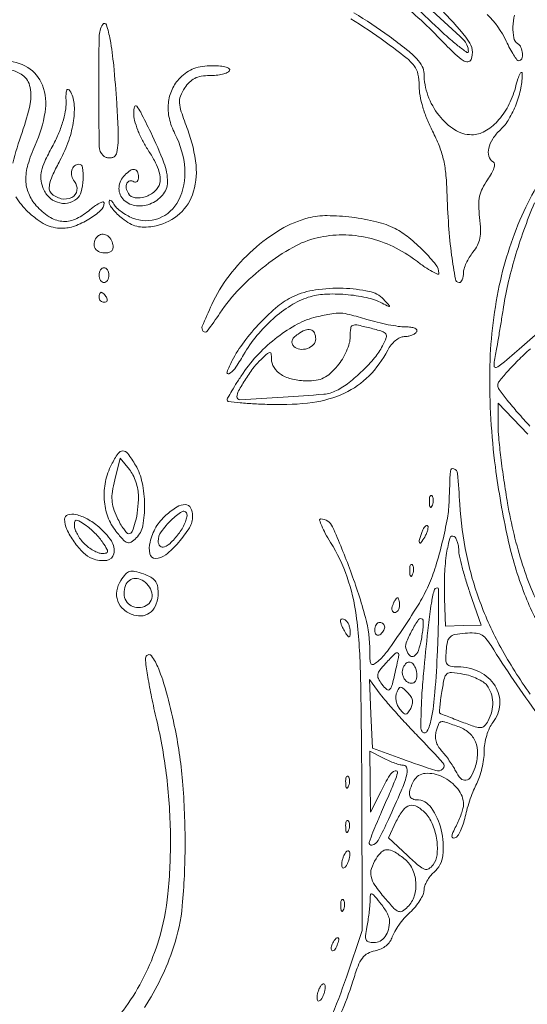
# Model space of a CAD drawing. Units: inches. Extents: x 2656 to 9931, y 1941 to 3068.
# Tile 38 of 46: x 2847 to 2854, y 2967 to 2981. Entities that reach past the tile are written whole.
import ezdxf

# ---------------------------------------------------------------- set-up
doc = ezdxf.new("R2010")
doc.units = ezdxf.units.IN
doc.layers.add('A-ANNO-DIMS', color=2, linetype='Continuous', lineweight=18)
doc.layers.add('A-ELEV-ORN', color=8, linetype='Continuous', lineweight=13)
doc.styles.get("Standard").update_dxf_attribs({"font": 'arial.ttf'})
doc.dimstyles.new('ISO-25', dxfattribs={"dimtxt": 6, "dimasz": 2.5, "dimexe": 1.25, "dimexo": 0.625, "dimtad": 1, "dimdec": 0, "dimlunit": 3, "dimtxsty": 'Standard', "dimcen": 2.5, "dimadec": 0, "dimazin": 0, "dimtfac": 1, "dimtdec": 0, "dimtmove": 0, "dimatfit": 3, "dimfxl": 1, "dimarcsym": 0})

# ---------------------------------------------------------------- blocks, each defined once
blk = doc.blocks.new('*D152')
at = {"layer": 'A-ANNO-DIMS', "color": 0, "lineweight": -2, "transparency": 16777216}
for p, q in [((2847.28, 2990.828), (2707.323, 2990.828)), ((2708.573, 2988.328), (2708.573, 2952.971)), ((2847.248, 2950.471), (2707.323, 2950.471))]:
    blk.add_line(p, q, dxfattribs=at)
at = {"layer": 'A-ANNO-DIMS', "color": 0, "transparency": 16777216}
for points in [[(2708.156, 2988.328), (2708.989, 2988.328), (2708.573, 2990.828)], [(2708.156, 2952.971), (2708.989, 2952.971), (2708.573, 2950.471)]]:
    blk.add_solid(points, dxfattribs=at)
at = {"layer": 'Defpoints', "color": 0, "transparency": 16777216}
for p in [(2847.905, 2990.828), (2708.573, 2950.471), (2847.873, 2950.471)]:
    blk.add_point(p, dxfattribs=at)
at = {"layer": 'A-ANNO-DIMS', "color": 0, "transparency": 16777216, "insert": (2704.843, 2970.649), "char_height": 6, "attachment_point": 5, "rotation": 90}
blk.add_mtext('3\'-4 1/2"', dxfattribs=at)
blk = doc.blocks.new('*D153')
at = {"layer": 'A-ANNO-DIMS', "color": 0, "lineweight": -2, "transparency": 16777216}
for p, q in [((2826.64, 2993.722), (2826.64, 2703.709)), ((2829.546, 2956.424), (2829.546, 2703.709)), ((2824.14, 2704.959), (2821.64, 2704.959)), ((2826.64, 2704.959), (2829.546, 2704.959)), ((2832.046, 2704.959), (2851.745, 2704.959))]:
    blk.add_line(p, q, dxfattribs=at)
at = {"layer": 'A-ANNO-DIMS', "color": 0, "transparency": 16777216}
for points in [[(2824.14, 2705.376), (2824.14, 2704.543), (2826.64, 2704.959)], [(2832.046, 2705.376), (2832.046, 2704.543), (2829.546, 2704.959)]]:
    blk.add_solid(points, dxfattribs=at)
at = {"layer": 'Defpoints', "color": 0, "transparency": 16777216}
for p in [(2826.64, 2994.347), (2829.546, 2957.049), (2829.546, 2704.959)]:
    blk.add_point(p, dxfattribs=at)
at = {"layer": 'A-ANNO-DIMS', "color": 0, "transparency": 16777216, "insert": (2843.145, 2708.65), "char_height": 6, "attachment_point": 5}
blk.add_mtext('0\'-3"', dxfattribs=at)
blk = doc.blocks.new('*D154')
at = {"layer": 'A-ANNO-DIMS', "color": 0, "lineweight": -2, "transparency": 16777216}
for p, q in [((2708.573, 2996.847), (2708.573, 2999.347)), ((2826.015, 2994.347), (2707.323, 2994.347)), ((2708.573, 2994.347), (2708.573, 2990.828)), ((2847.28, 2990.828), (2707.323, 2990.828)), ((2708.573, 2988.328), (2708.573, 2954.647))]:
    blk.add_line(p, q, dxfattribs=at)
at = {"layer": 'A-ANNO-DIMS', "color": 0, "transparency": 16777216}
for points in [[(2708.156, 2996.847), (2708.989, 2996.847), (2708.573, 2994.347)], [(2708.156, 2988.328), (2708.989, 2988.328), (2708.573, 2990.828)]]:
    blk.add_solid(points, dxfattribs=at)
at = {"layer": 'Defpoints', "color": 0, "transparency": 16777216}
for p in [(2826.64, 2994.347), (2708.573, 2990.828), (2847.905, 2990.828)]:
    blk.add_point(p, dxfattribs=at)
at = {"layer": 'A-ANNO-DIMS', "color": 0, "transparency": 16777216, "insert": (2704.843, 2970.237), "char_height": 6, "attachment_point": 5, "rotation": 90}
blk.add_mtext('0\'-3 1/2"', dxfattribs=at)

msp = doc.modelspace()

# ---------------------------------------------------------------- linework, layer by layer
at = {"layer": 'A-ELEV-ORN'}
for points in [[(2851.141, 2982.631, 0.234084), (2851.162, 2982.589, 0.005273), (2851.348, 2982.45, 0.010754), (2851.575, 2982.292, 0.006932), (2851.845, 2982.118, -0.022141), (2852.364, 2981.76, -0.017515), (2852.893, 2981.33, -0.010813), (2853.352, 2980.911, -0.205251), (2853.427, 2980.736, -0.610427), (2853.405, 2980.725, -0.012924), (2853.278, 2980.821, -0.01531), (2853.113, 2980.961, -0.008092), (2852.917, 2981.143, 0.023749), (2852.355, 2981.635, 0.02817), (2851.779, 2982.043, 0.029993), (2851.196, 2982.361, 0.036248), (2850.614, 2982.584), (2850.297, 2982.68), (2850.684, 2982.716, -0.006356), (2850.954, 2982.737, -0.06236), (2851.067, 2982.73, -0.194631), (2851.121, 2982.696, -0.155959)], [(2848.205, 2981.125, 0.135728), (2848.153, 2980.947, 0.004131), (2848.148, 2980.172, 0.003198), (2848.155, 2979.382, 0.194925), (2848.209, 2979.254, 0.091478), (2848.243, 2979.231, 0.076775), (2848.285, 2979.219, 0.07665), (2848.329, 2979.221, 0.090641), (2848.367, 2979.236, 0.211121), (2848.407, 2979.294, 0.03378), (2848.423, 2979.435, 0.023153), (2848.424, 2979.653, 0.006186), (2848.405, 2980, 0.00704), (2848.361, 2980.537, 0.020153), (2848.31, 2980.908, 0.035687), (2848.257, 2981.119, 0.637136)], [(2849.31, 2980.362, 0.089082), (2849.195, 2980.197, 0.084607), (2849.142, 2979.999, 0.078772), (2849.156, 2979.782, 0.063885), (2849.236, 2979.564, -0.100445), (2849.377, 2979.066, -0.136639), (2849.287, 2978.611, -0.186449), (2849.005, 2978.356, -0.192264), (2848.63, 2978.361, -0.032399), (2848.549, 2978.401, -0.028445), (2848.469, 2978.452, -0.029514), (2848.403, 2978.508, -0.072121), (2848.364, 2978.557, 0.029962), (2848.338, 2978.596, 0.125031), (2848.316, 2978.613, 0.364907), (2848.302, 2978.609, 0.143486), (2848.295, 2978.588, 0.146825), (2848.306, 2978.547, 0.031498), (2848.35, 2978.485, 0.030363), (2848.412, 2978.418, 0.024905), (2848.486, 2978.353, 0.038), (2848.592, 2978.282, 0.065429), (2848.69, 2978.243, 0.065493), (2848.795, 2978.23, 0.038149), (2848.922, 2978.241, 0.127134), (2849.27, 2978.393, 0.140443), (2849.485, 2978.691, 0.112579), (2849.537, 2979.114, 0.063942), (2849.419, 2979.619, -0.008179), (2849.326, 2979.879, -0.06362), (2849.301, 2980.005, -0.113197), (2849.316, 2980.102, -0.050089), (2849.376, 2980.218, -0.051689), (2849.444, 2980.301, -0.081241), (2849.519, 2980.355, -0.075737), (2849.612, 2980.385, -0.03941), (2849.732, 2980.394, 0.027097), (2849.827, 2980.399, 0.033643), (2849.915, 2980.415, 0.035766), (2849.984, 2980.437, 0.159159), (2850.016, 2980.465, 0.372154), (2850.012, 2980.493, 0.105375), (2849.969, 2980.516, 0.050611), (2849.887, 2980.53, 0.019267), (2849.771, 2980.535, 0.032494), (2849.625, 2980.525, 0.057102), (2849.508, 2980.496, 0.061656), (2849.407, 2980.443, 0.04528)], [(2847.681, 2980.016, -0.051991), (2847.67, 2979.882, -0.030277), (2847.632, 2979.726, -0.02723), (2847.569, 2979.555, -0.021618), (2847.483, 2979.378, 0.013301), (2847.376, 2979.168, 0.053097), (2847.329, 2979.032, 0.080458), (2847.321, 2978.92, 0.061642), (2847.347, 2978.799, 0.108477), (2847.429, 2978.666, 0.119741), (2847.558, 2978.585, 0.126458), (2847.703, 2978.574, 0.129345), (2847.835, 2978.635, 0.160352), (2847.896, 2978.733, 0.045574), (2847.924, 2978.913, 0.047035), (2847.918, 2979.081, 0.377174), (2847.864, 2979.128, 0.180978), (2847.8, 2979.104, 0.151421), (2847.762, 2979.042, 0.125839), (2847.761, 2978.959, 0.111844), (2847.801, 2978.882, -0.211931), (2847.836, 2978.756, -0.246157), (2847.764, 2978.656, -0.170782), (2847.611, 2978.637, -0.14386), (2847.467, 2978.716, -0.18574), (2847.441, 2978.775, -0.07904), (2847.45, 2978.863, -0.044281), (2847.497, 2978.991, -0.012123), (2847.594, 2979.183, 0.038511), (2847.72, 2979.47, 0.048655), (2847.788, 2979.752, 0.056214), (2847.796, 2979.998, 0.120966), (2847.736, 2980.177, 0.166742), (2847.71, 2980.197, 0.4182), (2847.69, 2980.188, 0.077929), (2847.68, 2980.131, 0.012295)], [(2848.647, 2979.861, 0.066256), (2848.66, 2979.754, 0.028758), (2848.704, 2979.617, 0.027029), (2848.771, 2979.47, 0.026615), (2848.853, 2979.33, -0.020796), (2848.942, 2979.182, -0.039929), (2848.999, 2979.055, -0.051296), (2849.025, 2978.948, -0.098566), (2849.02, 2978.86, -0.148842), (2848.948, 2978.743, -0.100958), (2848.81, 2978.663, -0.114169), (2848.666, 2978.65, -0.224679), (2848.571, 2978.711, -0.091812), (2848.541, 2978.789, -0.156827), (2848.549, 2978.858, -0.246696), (2848.591, 2978.89, -0.182491), (2848.649, 2978.879, 0.153598), (2848.674, 2978.873, 0.191518), (2848.696, 2978.883, 0.129571), (2848.71, 2978.909, 0.06068), (2848.715, 2978.948, 0.096897), (2848.7, 2979.022, 0.270548), (2848.66, 2979.054, 0.181077), (2848.598, 2979.039, 0.049135), (2848.518, 2978.973, 0.173404), (2848.437, 2978.803, 0.206144), (2848.491, 2978.635, 0.173837), (2848.662, 2978.539, 0.133555), (2848.877, 2978.56, 0.125211), (2849.059, 2978.688, 0.175896), (2849.129, 2978.873, 0.095151), (2849.079, 2979.15, 0.022174), (2848.89, 2979.585, 0.003547), (2848.747, 2979.871, 0.063293), (2848.69, 2979.956, 0.592353), (2848.659, 2979.949, 0.067838)], [(2851.141, 2978.362, 0.071146), (2850.745, 2978.197, 0.048928), (2850.353, 2977.909, 0.047402), (2850.01, 2977.537, 0.054543), (2849.762, 2977.124, 0.00865), (2849.627, 2976.817, 0.298499), (2849.641, 2976.743, 0.466073), (2849.698, 2976.747, 0.010316), (2849.878, 2977.002, -0.044182), (2850.166, 2977.358, -0.035773), (2850.532, 2977.685, -0.036975), (2850.919, 2977.942, -0.068908), (2851.269, 2978.078, -0.059555), (2851.629, 2978.121, -0.056517), (2851.996, 2978.078, -0.05503), (2852.353, 2977.952, -0.05102), (2852.684, 2977.75, 0.012612), (2852.807, 2977.66, 0.02442), (2852.911, 2977.596, 0.028666), (2852.987, 2977.56, 0.533446), (2853.005, 2977.572, 0.170044), (2852.963, 2977.694, 0.02544), (2852.788, 2977.891, 0.029403), (2852.578, 2978.082, 0.051547), (2852.38, 2978.21, 0.058451), (2852.116, 2978.308, 0.028989), (2851.763, 2978.372, 0.02895), (2851.409, 2978.395, 0.064691)], [(2848.13, 2978.098, 0.124772), (2848.085, 2978.022, 0.171832), (2848.089, 2977.943, 0.172015), (2848.142, 2977.884, 0.125046), (2848.228, 2977.862, 0.055584), (2848.291, 2977.869, 0.135583), (2848.332, 2977.891, 0.162135), (2848.351, 2977.928, 0.089805), (2848.351, 2977.979, 0.095165), (2848.318, 2978.061, 0.127216), (2848.259, 2978.116, 0.157051), (2848.191, 2978.128, 0.16545)], [(2848.152, 2977.546, 0.064853), (2848.157, 2977.505, 0.082425), (2848.173, 2977.471, 0.098894), (2848.196, 2977.448, 0.148195), (2848.223, 2977.44, 0.148195), (2848.249, 2977.448, 0.098894), (2848.272, 2977.471, 0.082425), (2848.288, 2977.505, 0.064853), (2848.293, 2977.546, 0.064853), (2848.288, 2977.586, 0.082425), (2848.272, 2977.62, 0.098894), (2848.249, 2977.643, 0.148195), (2848.223, 2977.651, 0.148195), (2848.196, 2977.643, 0.098894), (2848.173, 2977.62, 0.082425), (2848.157, 2977.586, 0.064853)], [(2848.152, 2977.229, 0.105053), (2848.158, 2977.202, 0.099167), (2848.174, 2977.18, 0.09642), (2848.198, 2977.164, 0.093332), (2848.227, 2977.159, 0.108972), (2848.252, 2977.164, 0.182303), (2848.267, 2977.18, 0.161196), (2848.269, 2977.202, 0.082592), (2848.258, 2977.229, 0.029505), (2848.239, 2977.256, 0.035638), (2848.218, 2977.279, 0.038439), (2848.198, 2977.295, 0.151918), (2848.183, 2977.3, 0.210953), (2848.171, 2977.294, 0.081139), (2848.161, 2977.279, 0.061769), (2848.154, 2977.256, 0.042167)], [(2850.925, 2977.24, 0.064367), (2850.705, 2977.101, 0.028896), (2850.456, 2976.867, 0.02857), (2850.223, 2976.593, 0.041883), (2850.055, 2976.326, 0.028815), (2849.98, 2976.161, 0.684631), (2850.008, 2976.136, 0.12746), (2850.09, 2976.209, 0.016725), (2850.216, 2976.408, -0.039198), (2850.407, 2976.682, -0.039456), (2850.638, 2976.923, -0.041641), (2850.89, 2977.111, -0.060325), (2851.141, 2977.229, -0.06635), (2851.374, 2977.273, -0.033594), (2851.673, 2977.269, -0.033577), (2851.97, 2977.225, -0.0641), (2852.196, 2977.144, 0.002728), (2852.29, 2977.097, 0.456781), (2852.3, 2977.1, 0.274534), (2852.297, 2977.114, 0.001926), (2852.215, 2977.2, 0.152232), (2852.009, 2977.314, 0.043207), (2851.641, 2977.358, 0.043501), (2851.243, 2977.335, 0.073803)], [(2851.256, 2976.948, 0.065131), (2850.984, 2976.845, 0.040432), (2850.698, 2976.66, 0.038683), (2850.429, 2976.419, 0.042607), (2850.21, 2976.146, 0.005701), (2850.122, 2976.013, 0.008315), (2850.048, 2975.893, 0.004667), (2849.989, 2975.791, 0.130083), (2849.981, 2975.762, 0.379498), (2849.997, 2975.743, 0.004803), (2850.166, 2975.724, 0.011035), (2850.37, 2975.708, 0.006661), (2850.613, 2975.698, 0.040601), (2851.202, 2975.728, 0.076164), (2851.658, 2975.861, 0.088703), (2852.008, 2976.107, 0.074925), (2852.275, 2976.473, -0.048849), (2852.324, 2976.548, -0.051822), (2852.386, 2976.611, -0.057407), (2852.451, 2976.653, -0.114934), (2852.511, 2976.667, 0.047477), (2852.565, 2976.672, 0.046582), (2852.619, 2976.687, 0.05048), (2852.662, 2976.71, 0.110322), (2852.689, 2976.737, 0.284272), (2852.689, 2976.764, 0.152033), (2852.662, 2976.787, 0.073352), (2852.607, 2976.802, 0.030038), (2852.528, 2976.807, -0.034672), (2852.426, 2976.814, -0.012452), (2852.283, 2976.838, -0.012283), (2852.126, 2976.872, -0.014243), (2851.979, 2976.912, 0.008231), (2851.73, 2976.983, 0.053096), (2851.601, 2977.003, 0.058929), (2851.477, 2976.995, 0.011461)], [(2852.2, 2976.535, -0.052361), (2852.088, 2976.366, -0.027521), (2851.916, 2976.18, -0.027428), (2851.723, 2976.012, -0.046222), (2851.542, 2975.897, -0.098221), (2851.363, 2975.845, -0.005454), (2850.78, 2975.803, -0.002477), (2850.165, 2975.767, -0.430285), (2850.122, 2975.808, -0.129249), (2850.144, 2975.892, -0.013881), (2850.248, 2976.064, -0.01802), (2850.366, 2976.234, -0.047813), (2850.466, 2976.343, -0.006806), (2850.56, 2976.426, -0.165761), (2850.592, 2976.439, -0.398077), (2850.61, 2976.424, -0.026675), (2850.614, 2976.351, 0.146923), (2850.651, 2976.227, 0.107386), (2850.755, 2976.126, 0.08407), (2850.916, 2976.059, 0.053851), (2851.118, 2976.036, 0.039919), (2851.254, 2976.045, 0.075755), (2851.36, 2976.078, 0.071847), (2851.454, 2976.142, 0.032774), (2851.557, 2976.25, 0.038586), (2851.628, 2976.348, 0.032848), (2851.686, 2976.461, 0.034177), (2851.726, 2976.572, 0.06942), (2851.739, 2976.664, -0.027223), (2851.746, 2976.787, -0.264388), (2851.775, 2976.828, -0.161063), (2851.836, 2976.834, -0.009463), (2852.018, 2976.792, -0.010674), (2852.197, 2976.742, -0.166952), (2852.248, 2976.706, -0.25386), (2852.254, 2976.653, -0.026234)], [(2851.247, 2976.635, -0.193252), (2851.214, 2976.554, -0.119848), (2851.127, 2976.498, -0.114454), (2851.02, 2976.487, -0.168464), (2850.936, 2976.528, -0.101963), (2850.909, 2976.57, -0.173175), (2850.908, 2976.611, -0.118812), (2850.935, 2976.654, -0.036758), (2850.994, 2976.704, -0.062759), (2851.094, 2976.76, -0.164638), (2851.175, 2976.765, -0.218499), (2851.228, 2976.721, -0.111164)], [(2848.33, 2974.841, 0.068391), (2848.244, 2974.598, 0.067917), (2848.226, 2974.34, 0.070296), (2848.278, 2974.094, 0.083269), (2848.394, 2973.888, 0.012798), (2848.5, 2973.763, 0.131333), (2848.557, 2973.727, 0.229197), (2848.609, 2973.734, 0.047917), (2848.683, 2973.793, 0.153704), (2848.776, 2973.968, 0.048813), (2848.802, 2974.266, 0.048367), (2848.768, 2974.583, 0.082752), (2848.673, 2974.831, 0.023094), (2848.563, 2974.998, 0.232629), (2848.492, 2975.036, 0.258719), (2848.424, 2975, 0.027881)], [(2848.714, 2974.39, -0.026627), (2848.703, 2974.193, -0.035986), (2848.67, 2974.018, -0.037978), (2848.625, 2973.887, -0.299568), (2848.574, 2973.853, -0.218414), (2848.547, 2973.866, -0.023577), (2848.504, 2973.921, -0.025504), (2848.456, 2973.996, -0.017827), (2848.41, 2974.085, -0.033622), (2848.358, 2974.217, -0.062504), (2848.337, 2974.331, -0.055489), (2848.343, 2974.455, -0.02145), (2848.378, 2974.623), (2848.456, 2974.931), (2848.586, 2974.771, -0.055401), (2848.635, 2974.694, -0.033509), (2848.677, 2974.593, -0.033255), (2848.705, 2974.487, -0.049208)], [(2852.87, 2974.304, 0.018894), (2852.874, 2974.252, 0.168741), (2852.884, 2974.231, 0.470617), (2852.897, 2974.233, 0.054073), (2852.913, 2974.262, 0.051402), (2852.924, 2974.3, 0.05415), (2852.926, 2974.34, 0.060344), (2852.921, 2974.374, 0.126455), (2852.907, 2974.397, 0.296942), (2852.892, 2974.4, 0.208169), (2852.879, 2974.387, 0.077125), (2852.871, 2974.353, 0.028489)], [(2849.106, 2974.117, 0.080088), (2848.964, 2973.946, 0.074133), (2848.88, 2973.734, 0.112243), (2848.878, 2973.567, 0.352942), (2848.959, 2973.501, 0.171195), (2849.105, 2973.553, 0.04353), (2849.289, 2973.73, 0.044193), (2849.442, 2973.939, 0.136315), (2849.489, 2974.107, 0.121461), (2849.46, 2974.223, 0.271607), (2849.385, 2974.269, 0.148417), (2849.266, 2974.237, 0.039714)], [(2849.299, 2973.868, -0.031591), (2849.183, 2973.731, -0.104818), (2849.086, 2973.665, -0.298481), (2849.025, 2973.677, -0.201654), (2848.996, 2973.745, -0.155884), (2849.04, 2973.881, -0.044757), (2849.185, 2974.05, -0.055079), (2849.335, 2974.168, -0.483759), (2849.404, 2974.143, -0.132295), (2849.407, 2974.095, -0.039811), (2849.386, 2974.024, -0.036815), (2849.349, 2973.944, -0.032661)], [(2847.66, 2974.061, 0.110949), (2847.692, 2973.916, 0.04287), (2847.796, 2973.738, 0.042914), (2847.929, 2973.58, 0.106036), (2848.056, 2973.498, 0.120781), (2848.262, 2973.473, 0.324755), (2848.364, 2973.567, 0.199087), (2848.328, 2973.75, 0.070743), (2848.147, 2973.952, 0.04832), (2847.983, 2974.065, 0.072026), (2847.821, 2974.126, 0.126394), (2847.706, 2974.123, 0.333237)], [(2848.208, 2973.725, -0.011478), (2848.265, 2973.635, -0.156567), (2848.274, 2973.597, -0.338836), (2848.256, 2973.577, -0.045786), (2848.196, 2973.572, -0.090506), (2848.142, 2973.582, -0.035885), (2848.074, 2973.613, -0.034042), (2848.003, 2973.659, -0.036207), (2847.941, 2973.712, -0.036207), (2847.887, 2973.775, -0.034042), (2847.842, 2973.845, -0.035885), (2847.81, 2973.914, -0.090506), (2847.801, 2973.967, -0.045786), (2847.806, 2974.027, -0.338836), (2847.826, 2974.045, -0.156567), (2847.863, 2974.037, -0.011478), (2847.954, 2973.98, -0.031065), (2848.02, 2973.93, -0.018762), (2848.092, 2973.863, -0.018762), (2848.158, 2973.791, -0.031065)], [(2852.768, 2973.886, 0.013074), (2852.727, 2973.769, 0.18392), (2852.729, 2973.726, 0.582659), (2852.75, 2973.724, 0.022794), (2852.803, 2973.806, 0.028467), (2852.829, 2973.857, 0.039963), (2852.846, 2973.906, 0.045448), (2852.852, 2973.946, 0.217548), (2852.845, 2973.967, 0.299281), (2852.829, 2973.97, 0.109577), (2852.808, 2973.957, 0.064271), (2852.787, 2973.927, 0.033338)], [(2853.29, 2973.62, 0.050057), (2853.3, 2973.534, 0.00925), (2853.338, 2973.377, 0.009843), (2853.39, 2973.194, 0.008828), (2853.45, 2973.008), (2853.608, 2972.549), (2853.354, 2972.542), (2853.1, 2972.535), (2853.087, 2972.931, -0.018117), (2853.088, 2973.279, -0.028041), (2853.117, 2973.578, -0.030846), (2853.164, 2973.791, -0.498245), (2853.223, 2973.814, -0.126966), (2853.247, 2973.788, -0.044697), (2853.269, 2973.741, -0.040881), (2853.284, 2973.682, -0.037663)], [(2848.463, 2973.186, 0.105069), (2848.406, 2973.038, 0.130425), (2848.42, 2972.892, 0.128099), (2848.506, 2972.77, 0.099419), (2848.648, 2972.692, 0.121082), (2848.781, 2972.683, 0.14276), (2848.895, 2972.739, 0.125398), (2848.97, 2972.854, 0.082675), (2848.996, 2973.011, 0.052324), (2848.986, 2973.112, 0.114745), (2848.953, 2973.181, 0.10422), (2848.89, 2973.234, 0.038494), (2848.785, 2973.28, 0.027034), (2848.662, 2973.316, 0.128575), (2848.59, 2973.313, 0.141997), (2848.532, 2973.277, 0.035606)], [(2852.589, 2973.32, 0.018894), (2852.593, 2973.267, 0.168741), (2852.603, 2973.247, 0.470617), (2852.616, 2973.248, 0.054073), (2852.631, 2973.277, 0.051402), (2852.642, 2973.316, 0.05415), (2852.645, 2973.355, 0.060344), (2852.639, 2973.389, 0.126455), (2852.626, 2973.412, 0.296942), (2852.61, 2973.415, 0.208169), (2852.597, 2973.402, 0.077125), (2852.59, 2973.369, 0.028489)], [(2848.855, 2973.116, -0.11992), (2848.906, 2973.01, -0.158954), (2848.896, 2972.904, -0.163385), (2848.825, 2972.827, -0.127627), (2848.715, 2972.798, -0.123681), (2848.612, 2972.824, -0.137936), (2848.539, 2972.895, -0.127411), (2848.509, 2972.998, -0.097756), (2848.529, 2973.115, -0.142834), (2848.585, 2973.188, -0.159877), (2848.67, 2973.216, -0.132962), (2848.766, 2973.19, -0.088248)], [(2852.986, 2972.183, -0.008133), (2852.949, 2971.591, -0.027669), (2852.898, 2971.207, -0.076068), (2852.836, 2971.031, -0.577831), (2852.766, 2971.029, -0.141413), (2852.748, 2971.092, -0.005787), (2852.753, 2971.33, -0.009694), (2852.767, 2971.616, -0.006683), (2852.794, 2971.938, -0.002281), (2852.857, 2972.549, -0.014195), (2852.899, 2972.861, -0.020173), (2852.937, 2973.044, -0.344538), (2852.982, 2973.079, -0.410173), (2852.999, 2973.062, -0.002399), (2853.002, 2972.816, -0.007747), (2852.998, 2972.527, -0.004637)], [(2852.347, 2972.833, 0.055937), (2852.336, 2972.793, 0.100118), (2852.338, 2972.759, 0.147206), (2852.352, 2972.736, 0.184534), (2852.375, 2972.728, 0.152681), (2852.4, 2972.736, 0.098158), (2852.423, 2972.759, 0.08088), (2852.438, 2972.793, 0.062722), (2852.443, 2972.833, 0.024748), (2852.441, 2972.874, 0.039339), (2852.435, 2972.908, 0.046727), (2852.426, 2972.932, 0.289661), (2852.415, 2972.939, 0.222225), (2852.402, 2972.933, 0.030693), (2852.384, 2972.908, 0.030395), (2852.364, 2972.874, 0.02136)], [(2851.6, 2972.609, 0.074451), (2851.605, 2972.58, 0.021733), (2851.62, 2972.538, 0.021318), (2851.643, 2972.491, 0.021347), (2851.669, 2972.446, 0.010223), (2851.709, 2972.387, 0.295079), (2851.725, 2972.381, 0.343021), (2851.736, 2972.393, 0.012098), (2851.738, 2972.46, 0.053738), (2851.733, 2972.509, 0.049393), (2851.718, 2972.557, 0.052761), (2851.696, 2972.597, 0.101161), (2851.669, 2972.622, 0.058538), (2851.642, 2972.635, 0.128516), (2851.62, 2972.636, 0.195945), (2851.605, 2972.627, 0.157323)], [(2852.756, 2972.348, -0.03519), (2852.713, 2972.186, -0.157554), (2852.655, 2972.107, -0.361972), (2852.595, 2972.112, -0.109119), (2852.541, 2972.195, -0.184366), (2852.54, 2972.295, -0.031567), (2852.621, 2972.472, -0.032288), (2852.716, 2972.627, -0.464078), (2852.773, 2972.632, -0.199934), (2852.783, 2972.608, -0.014301), (2852.781, 2972.536, -0.018345), (2852.772, 2972.447, -0.012736)], [(2852.091, 2972.477, 0.066118), (2852.096, 2972.439, 0.138808), (2852.112, 2972.413, 0.191142), (2852.135, 2972.404, 0.139169), (2852.161, 2972.411, 0.06081), (2852.188, 2972.433, 0.051032), (2852.211, 2972.461, 0.053229), (2852.226, 2972.492, 0.089642), (2852.232, 2972.521, 0.105429), (2852.226, 2972.546, 0.099231), (2852.211, 2972.568, 0.096318), (2852.188, 2972.582, 0.092995), (2852.161, 2972.587, 0.153634), (2852.134, 2972.579, 0.097988), (2852.112, 2972.555, 0.080552), (2852.096, 2972.519, 0.062283)], [(2852.403, 2971.972, -0.005605), (2852.342, 2971.708, -0.107759), (2852.306, 2971.633, -0.42445), (2852.262, 2971.629, -0.058569), (2852.192, 2971.704, -0.043651), (2852.142, 2971.785, -0.159754), (2852.133, 2971.844, -0.12386), (2852.161, 2971.906, -0.021894), (2852.244, 2972.002, -0.006044), (2852.378, 2972.141, -0.251072), (2852.416, 2972.153, -0.40947), (2852.434, 2972.127, -0.010104)], [(2852.671, 2971.937, -0.077734), (2852.692, 2971.83, -0.156942), (2852.67, 2971.748, -0.258961), (2852.614, 2971.719, -0.168914), (2852.545, 2971.745, -0.076541), (2852.512, 2971.783, -0.067375), (2852.49, 2971.83, -0.069989), (2852.482, 2971.88, -0.097891), (2852.49, 2971.924, -0.08069), (2852.53, 2971.994, -0.206319), (2852.582, 2972.021, -0.22957), (2852.632, 2972.001, -0.096355)], [(2852.751, 2970.917, -0.009029), (2853.063, 2970.583, -0.39704), (2853.061, 2970.495, -0.286499), (2852.96, 2970.471, -0.006735), (2852.478, 2970.64), (2852.056, 2970.794), (2852.035, 2971.282), (2852.014, 2971.771), (2852.169, 2971.564, 0.017682), (2852.256, 2971.456, 0.004597), (2852.404, 2971.288, 0.004668), (2852.576, 2971.1, 0.004751)], [(2853.691, 2971.69, -0.080224), (2853.751, 2971.578, -0.074911), (2853.775, 2971.45, -0.070955), (2853.761, 2971.315, -0.06095), (2853.709, 2971.181, -0.064122), (2853.659, 2971.11, -0.196618), (2853.606, 2971.086, -0.093548), (2853.526, 2971.097, -0.008854), (2853.34, 2971.164, -0.001349), (2853.224, 2971.208, -0.002024), (2853.123, 2971.248, -0.000813), (2853.036, 2971.282, -0.045405), (2853.021, 2971.29, -0.276784), (2853.014, 2971.303, -0.004857), (2853.02, 2971.386, -0.010702), (2853.031, 2971.484, -0.00674), (2853.048, 2971.599, -0.013206), (2853.084, 2971.791, -0.167669), (2853.121, 2971.853, -0.200608), (2853.186, 2971.873, -0.020149), (2853.349, 2971.85, -0.033584), (2853.453, 2971.824, -0.031559), (2853.554, 2971.784, -0.033099), (2853.64, 2971.737, -0.086626)], [(2852.603, 2971.359, -0.026458), (2852.562, 2971.295, -0.229289), (2852.534, 2971.279, -0.213121), (2852.502, 2971.291, -0.022844), (2852.447, 2971.351, -0.069718), (2852.416, 2971.401, -0.055025), (2852.397, 2971.463, -0.056271), (2852.391, 2971.525, -0.084195), (2852.402, 2971.579, -0.030212), (2852.432, 2971.645, -0.263445), (2852.458, 2971.661, -0.195222), (2852.491, 2971.65, -0.016857), (2852.558, 2971.587, -0.051748), (2852.605, 2971.53, -0.096337), (2852.627, 2971.475, -0.105385), (2852.626, 2971.419, -0.071281)], [(2853.277, 2971.103, -0.092049), (2853.431, 2971.015, -0.118685), (2853.528, 2970.883, -0.109657), (2853.558, 2970.713, -0.070252), (2853.522, 2970.515, -0.051377), (2853.462, 2970.382, -0.221202), (2853.393, 2970.334, -0.257641), (2853.319, 2970.36, -0.065779), (2853.245, 2970.467, 0.022081), (2853.207, 2970.534, 0.012259), (2853.155, 2970.613, 0.012207), (2853.098, 2970.69, 0.01926), (2853.045, 2970.753, -0.052153), (2852.996, 2970.82, -0.065254), (2852.966, 2970.892, -0.069856), (2852.957, 2970.964, -0.073848), (2852.969, 2971.035, -0.018308), (2853.007, 2971.143, -0.247872), (2853.038, 2971.169, -0.134828), (2853.088, 2971.167, -0.004424)], [(2852.5, 2970.548, -0.369244), (2852.55, 2970.505, -0.105886), (2852.543, 2970.395, -0.034656), (2852.468, 2970.183, -0.005305), (2852.285, 2969.774, -0.014101), (2852.138, 2969.475, -0.211347), (2852.049, 2969.405, -0.599873), (2852.011, 2969.447, -0.017019), (2852.122, 2969.732, -0.000025), (2852.172, 2969.847, -0.000015), (2852.231, 2969.983, -0.000015), (2852.289, 2970.118, -0.000026), (2852.338, 2970.231, 0.023668), (2852.416, 2970.437, 0.614977), (2852.383, 2970.47, 0.181406), (2852.303, 2970.406, 0.016573), (2852.18, 2970.178), (2852.029, 2969.879), (2852.025, 2970.315), (2852.021, 2970.75), (2852.214, 2970.649, 0.017428), (2852.295, 2970.611, 0.017675), (2852.378, 2970.578, 0.017762), (2852.452, 2970.555, 0.066272)], [(2851.675, 2970.295, 0.018894), (2851.679, 2970.243, 0.168741), (2851.689, 2970.222, 0.470617), (2851.701, 2970.224, 0.054073), (2851.717, 2970.253, 0.051402), (2851.728, 2970.291, 0.05415), (2851.731, 2970.331, 0.060344), (2851.725, 2970.365, 0.126455), (2851.711, 2970.388, 0.296942), (2851.696, 2970.391, 0.208169), (2851.683, 2970.378, 0.077125), (2851.675, 2970.344, 0.028489)], [(2852.822, 2969.853, -0.091293), (2852.921, 2969.692, -0.058457), (2852.976, 2969.479, -0.060377), (2852.98, 2969.27, -0.139497), (2852.922, 2969.126, -0.08943), (2852.86, 2969.07, -0.229662), (2852.802, 2969.064, -0.091555), (2852.723, 2969.11, -0.008765), (2852.557, 2969.258), (2852.284, 2969.51), (2852.398, 2969.748, -0.048684), (2852.494, 2969.908, -0.173694), (2852.592, 2969.973, -0.203558), (2852.699, 2969.956, -0.068936)], [(2851.675, 2969.662, 0.018894), (2851.679, 2969.61, 0.168741), (2851.689, 2969.589, 0.470617), (2851.701, 2969.591, 0.054073), (2851.717, 2969.62, 0.051402), (2851.728, 2969.658, 0.05415), (2851.731, 2969.698, 0.060344), (2851.725, 2969.732, 0.126455), (2851.711, 2969.755, 0.296942), (2851.696, 2969.758, 0.208169), (2851.683, 2969.745, 0.077125), (2851.675, 2969.711, 0.028489)], [(2851.641, 2969.239, 0.033304), (2851.626, 2969.191, 0.041541), (2851.619, 2969.145, 0.04665), (2851.62, 2969.107, 0.168083), (2851.63, 2969.085, 0.291964), (2851.648, 2969.082, 0.11331), (2851.669, 2969.095, 0.066301), (2851.691, 2969.126, 0.03436), (2851.711, 2969.169, 0.033304), (2851.726, 2969.217, 0.041541), (2851.733, 2969.263, 0.04665), (2851.732, 2969.301, 0.168083), (2851.721, 2969.323, 0.291964), (2851.704, 2969.326, 0.11331), (2851.683, 2969.313, 0.066301), (2851.661, 2969.282, 0.03436)], [(2852.507, 2969.218, -0.11749), (2852.624, 2969.074, -0.093162), (2852.676, 2968.879, -0.093956), (2852.654, 2968.681, -0.122278), (2852.56, 2968.525, -0.060462), (2852.486, 2968.466, -0.232687), (2852.429, 2968.462, -0.113215), (2852.364, 2968.505, -0.010495), (2852.235, 2968.651, -0.022515), (2852.092, 2968.834, -0.099108), (2852.037, 2968.958, -0.136844), (2852.042, 2969.073, -0.059146), (2852.108, 2969.212, -0.062596), (2852.188, 2969.31, -0.189123), (2852.266, 2969.342, -0.139289), (2852.362, 2969.317, -0.029164)], [(2852.302, 2968.33, -0.060826), (2852.286, 2968.202, -0.096021), (2852.24, 2968.101, -0.115815), (2852.167, 2968.038, -0.121512), (2852.075, 2968.015, -0.064174), (2852.001, 2968.025, -0.227594), (2851.966, 2968.055, -0.135761), (2851.957, 2968.113, -0.019247), (2851.977, 2968.235, 0.01022), (2851.994, 2968.33, 0.007946), (2852.008, 2968.434, 0.008046), (2852.019, 2968.532, 0.019227), (2852.023, 2968.604, -0.013513), (2852.027, 2968.699, -0.428239), (2852.043, 2968.712, -0.187426), (2852.07, 2968.698, -0.004437), (2852.164, 2968.588, -0.024625), (2852.217, 2968.518, -0.025996), (2852.261, 2968.444, -0.026794), (2852.293, 2968.376, -0.096548)], [(2851.604, 2968.537, 0.018894), (2851.608, 2968.485, 0.168741), (2851.618, 2968.464, 0.470617), (2851.631, 2968.465, 0.054073), (2851.647, 2968.495, 0.051402), (2851.658, 2968.533, 0.05415), (2851.66, 2968.572, 0.060344), (2851.655, 2968.606, 0.126455), (2851.641, 2968.629, 0.296942), (2851.626, 2968.633, 0.208169), (2851.613, 2968.62, 0.077125), (2851.605, 2968.586, 0.028489)], [(2851.49, 2968.011, 0.049364), (2851.475, 2967.98, 0.059701), (2851.467, 2967.948, 0.070517), (2851.468, 2967.921, 0.156651), (2851.477, 2967.902, 0.281567), (2851.493, 2967.898, 0.118528), (2851.513, 2967.91, 0.069269), (2851.534, 2967.938, 0.035865), (2851.553, 2967.977, 0.029555), (2851.577, 2968.055, 0.344086), (2851.565, 2968.082, 0.36195), (2851.537, 2968.077, 0.030391)], [(2851.289, 2967.34, 0.033304), (2851.274, 2967.292, 0.041541), (2851.267, 2967.246, 0.04665), (2851.268, 2967.208, 0.168083), (2851.279, 2967.186, 0.291964), (2851.296, 2967.183, 0.11331), (2851.317, 2967.196, 0.066301), (2851.34, 2967.227, 0.03436), (2851.359, 2967.27, 0.033304), (2851.374, 2967.318, 0.041541), (2851.381, 2967.364, 0.04665), (2851.38, 2967.402, 0.168083), (2851.37, 2967.424, 0.291964), (2851.353, 2967.427, 0.11331), (2851.332, 2967.414, 0.066301), (2851.309, 2967.383, 0.03436)]]:
    msp.add_lwpolyline(points, format="xyb", close=True, dxfattribs=at)
for points in [[(2852.373, 2981.502, -0.036376), (2853.026, 2980.915, 0.00697), (2853.238, 2980.7, 0.048733), (2853.353, 2980.608, 0.169575), (2853.421, 2980.59, 0.286241), (2853.466, 2980.625, 0.256031), (2853.43, 2980.888, 0.039762), (2853.073, 2981.299, 0.035403)], [(2851.747, 2981.205, -0.019692), (2852.24, 2980.876, -0.007963), (2852.534, 2980.654, -0.063825), (2852.653, 2980.534, -0.114572), (2852.707, 2980.417, -0.049754), (2852.724, 2980.246, 0.046764), (2852.737, 2980.108, 0.025261), (2852.777, 2979.943, 0.023865), (2852.838, 2979.768, 0.024156), (2852.915, 2979.601, -0.024979), (2853.009, 2979.396, -0.036323), (2853.069, 2979.207, -0.033608), (2853.104, 2979.001, -0.017716), (2853.121, 2978.741, 0.010302), (2853.145, 2978.253, 0.015669), (2853.188, 2977.831, 0.009059), (2853.241, 2977.486, 0.365327), (2853.295, 2977.44, 0.202945), (2853.319, 2977.45, 0.084109), (2853.339, 2977.479, 0.064256), (2853.352, 2977.522, 0.044424), (2853.357, 2977.573, -0.074784), (2853.366, 2977.636, -0.03139), (2853.397, 2977.716, -0.030182), (2853.44, 2977.799, -0.034442), (2853.492, 2977.872, 0.051894), (2853.557, 2977.971, 0.070715), (2853.591, 2978.071, 0.056292), (2853.601, 2978.194, 0.021188), (2853.588, 2978.366, -0.023096), (2853.576, 2978.543, -0.057537), (2853.588, 2978.671, -0.06552), (2853.627, 2978.784, -0.037959), (2853.701, 2978.906, 0.025243), (2853.759, 2978.997, 0.054404), (2853.792, 2979.073, 0.084167), (2853.799, 2979.13, 0.250492), (2853.78, 2979.163, -0.187184), (2853.72, 2979.242, -0.12591), (2853.717, 2979.357, -0.090788), (2853.775, 2979.491, -0.057687), (2853.885, 2979.621, 0.071523), (2854.006, 2979.773, 0.040925), (2854.109, 2979.986, 0.040406), (2854.177, 2980.218, 0.059271), (2854.196, 2980.429, 0.453324), (2854.183, 2980.44, 0.247004), (2854.165, 2980.426, 0.034219), (2854.134, 2980.347, 0.010134), (2854.098, 2980.221, -0.055078), (2853.995, 2979.958, -0.066795), (2853.842, 2979.742, -0.077406), (2853.661, 2979.599, -0.128885), (2853.474, 2979.55, -0.142622), (2853.232, 2979.621, -0.085579), (2853.008, 2979.824, -0.078484), (2852.849, 2980.111, -0.087561), (2852.794, 2980.422, 0.125398), (2852.768, 2980.524, 0.06277), (2852.689, 2980.634, 0.037669), (2852.544, 2980.768, 0.010404), (2852.297, 2980.956, 0.020948), (2851.793, 2981.291, 0.02459)], [(2853.697, 2981.268, -0.092556), (2853.968, 2980.885, 0.014479), (2854.021, 2980.779, 0.021232), (2854.074, 2980.689, 0.017507), (2854.121, 2980.621, 0.226696), (2854.148, 2980.607, 0.323525), (2854.189, 2980.634, 0.106759), (2854.199, 2980.709, 0.084043), (2854.178, 2980.797, 0.153694), (2854.131, 2980.851, -0.21056), (2854.076, 2980.932, -0.053676), (2854.063, 2981.092, -0.053592), (2854.085, 2981.259, -0.136805)], [(2846.962, 2978.664, 0.063929), (2847.137, 2978.451, 0.026315), (2847.267, 2978.341, 0.048737), (2847.384, 2978.269, 0.057356), (2847.499, 2978.228, 0.056794), (2847.62, 2978.214, 0.087216), (2847.803, 2978.246, 0.048646), (2848.007, 2978.344, 0.048421), (2848.174, 2978.467, 0.211797), (2848.223, 2978.577, 0.48043), (2848.206, 2978.59, 0.064732), (2848.157, 2978.572, 0.037306), (2848.086, 2978.528, 0.017778), (2848, 2978.461, -0.073901), (2847.807, 2978.342, -0.127031), (2847.621, 2978.314, -0.121499), (2847.438, 2978.379, -0.06433), (2847.255, 2978.537, -0.082793), (2847.147, 2978.709, -0.095342), (2847.106, 2978.899, -0.076313), (2847.136, 2979.123, -0.03499), (2847.239, 2979.4, 0.06686), (2847.381, 2979.87, 0.129555), (2847.343, 2980.258, 0.170204), (2847.133, 2980.51, 0.135833), (2846.791, 2980.605, -0.034455)], [(2846.802, 2980.495, -0.106727), (2847.038, 2980.415, -0.193218), (2847.16, 2980.255, -0.120182), (2847.168, 2979.991, -0.031739), (2847.053, 2979.582, 0.019278), (2846.919, 2979.144, 0.083581)], [(2854.772, 2979.332, 0.06803), (2854.218, 2978.456, 0.054859), (2853.869, 2977.398, 0.049024), (2853.733, 2976.174, 0.035727), (2853.813, 2974.807, 0.02083), (2853.99, 2973.788, 0.039593), (2854.23, 2972.992, 0.048806), (2854.547, 2972.366, 0.063105)], [(2854.616, 2976.893), (2854.189, 2976.521, -0.002591), (2853.907, 2976.278, -0.07477), (2853.826, 2976.228, -0.53609), (2853.794, 2976.248, -0.052978), (2853.805, 2976.356, 0.006919), (2853.826, 2976.466, 0.001808), (2853.856, 2976.644, 0.001837), (2853.89, 2976.846, 0.001879), (2853.922, 2977.048, -0.018186), (2853.991, 2977.412, -0.015083), (2854.091, 2977.794, -0.014514), (2854.219, 2978.186, -0.013623), (2854.371, 2978.577, -0.060131)], [(2854.306, 2975.391, -0.009083), (2854.131, 2975.583, -0.012896), (2853.983, 2975.761, -0.008942), (2853.867, 2975.913, -0.153971), (2853.847, 2975.972, -0.177904), (2853.867, 2976.029, -0.011192), (2853.983, 2976.165, -0.015374), (2854.134, 2976.325, -0.010744), (2854.313, 2976.495)], [(2854.521, 2972.659, -0.047105), (2854.202, 2973.409, -0.034503), (2853.987, 2974.288, -0.006153), (2853.935, 2974.616, -0.006266), (2853.891, 2974.943, -0.006108), (2853.86, 2975.228, -0.025672), (2853.852, 2975.4), (2853.854, 2975.717), (2854.274, 2975.276, -0.008047)], [(2854.308, 2971.564, -0.028331), (2853.89, 2972.23, -0.037211), (2853.592, 2972.884, -0.038525), (2853.401, 2973.555, -0.034121), (2853.305, 2974.275, 0.00609), (2853.271, 2974.714, 0.289642), (2853.22, 2974.782, 0.505023), (2853.17, 2974.749, 0.006969), (2853.153, 2974.331, -0.037407), (2853.127, 2974.075, -0.015466), (2853.055, 2973.734, -0.015571), (2852.96, 2973.389, -0.028284), (2852.857, 2973.115, -0.032995), (2852.727, 2972.864, -0.010771), (2852.503, 2972.513, -0.009044), (2852.27, 2972.176, -0.063373), (2852.134, 2972.031, -0.042719), (2852.07, 2971.987, -0.37381), (2852.04, 2971.993, -0.156582), (2852.023, 2972.037, -0.01014), (2852.021, 2972.175, 0.065774), (2851.957, 2972.659, 0.023456), (2851.744, 2973.322, 0.015416), (2851.487, 2973.954, 0.296403), (2851.317, 2974.064, 0.502654), (2851.303, 2974.046, 0.027241), (2851.332, 2973.966, 0.02478), (2851.384, 2973.858, 0.013161), (2851.459, 2973.73, -0.054593), (2851.695, 2973.235, -0.051145), (2851.824, 2972.689, -0.027256), (2851.885, 2971.882, -0.004613), (2851.904, 2970.336), (2851.91, 2968.191), (2851.685, 2967.523, -0.020457), (2851.452, 2966.917, -0.026412)], [(2851.598, 2966.989, 0.02788), (2851.777, 2967.464, -0.014526), (2851.851, 2967.68, -0.067426), (2851.914, 2967.796, -0.110097), (2851.989, 2967.862, -0.075939), (2852.096, 2967.9, 0.056638), (2852.18, 2967.927, 0.06434), (2852.252, 2967.972, 0.068179), (2852.307, 2968.03, 0.077771), (2852.341, 2968.099, -0.057206), (2852.375, 2968.173, -0.022763), (2852.436, 2968.267, -0.022171), (2852.512, 2968.363, -0.025962), (2852.593, 2968.447, 0.031725), (2852.67, 2968.528, 0.032826), (2852.735, 2968.618, 0.034757), (2852.781, 2968.703, 0.105981), (2852.794, 2968.766, -0.084636), (2852.804, 2968.826, -0.042691), (2852.836, 2968.895, -0.040785), (2852.881, 2968.963, -0.047849), (2852.935, 2969.019, 0.191421), (2853.062, 2969.261, 0.086233), (2853.038, 2969.626, 0.091749), (2852.896, 2969.943, 0.246549), (2852.684, 2970.055, -0.150861), (2852.619, 2970.075, -0.215557), (2852.588, 2970.126, -0.117608), (2852.597, 2970.211, -0.036454), (2852.65, 2970.329, -0.261585), (2852.811, 2970.432, -0.127577), (2853.057, 2970.383, -0.108135), (2853.277, 2970.209, -0.174847), (2853.357, 2969.987, -0.061961), (2853.35, 2969.932, -0.019052), (2853.326, 2969.852, -0.018741), (2853.292, 2969.764, -0.019514), (2853.252, 2969.68, 0.013937), (2853.207, 2969.587, 0.081369), (2853.193, 2969.534, 0.312065), (2853.205, 2969.512, 0.196844), (2853.235, 2969.51, 0.168309), (2853.273, 2969.538, 0.034684), (2853.314, 2969.611, 0.032885), (2853.352, 2969.707, 0.025813), (2853.382, 2969.814, -0.017802), (2853.412, 2969.934, -0.012466), (2853.455, 2970.068, -0.012597), (2853.502, 2970.193, -0.025494), (2853.547, 2970.289, 0.041916), (2853.587, 2970.383, 0.023135), (2853.621, 2970.504, 0.02292), (2853.645, 2970.631, 0.033943), (2853.652, 2970.744, -0.041681), (2853.662, 2970.854, -0.031453), (2853.689, 2970.972, -0.032183), (2853.729, 2971.08, -0.061435), (2853.777, 2971.159, 0.152691), (2853.876, 2971.417, 0.156945), (2853.808, 2971.682, 0.139015), (2853.587, 2971.88, 0.113081), (2853.277, 2971.953, -0.039354), (2853.174, 2971.962, -0.196784), (2853.125, 2971.992, -0.155667), (2853.105, 2972.052, -0.022439), (2853.11, 2972.183, -0.032073), (2853.128, 2972.314, -0.155353), (2853.165, 2972.378, -0.141702), (2853.234, 2972.413, -0.02515), (2853.379, 2972.433, -0.031728), (2853.516, 2972.436, -0.100091), (2853.606, 2972.414, -0.106331), (2853.677, 2972.36, -0.038416), (2853.752, 2972.257, 0.021715), (2854.422, 2971.271, 0.060142)], [(2848.802, 2967.089, 0.062193), (2849.216, 2967.949, 0.059261), (2849.341, 2968.542, 0.021327), (2849.381, 2969.405, 0.021471), (2849.344, 2970.323, 0.0321), (2849.227, 2971.117, 0.012043), (2849.112, 2971.596, 0.031282), (2849, 2971.932, 0.061667), (2848.902, 2972.108, 0.532561), (2848.827, 2972.106, 0.173915), (2848.814, 2972.045, 0.006183), (2848.85, 2971.806, 0.010774), (2848.902, 2971.521, 0.007264), (2848.973, 2971.199, -0.029103), (2849.118, 2970.377, -0.026423), (2849.172, 2969.517, -0.027576), (2849.135, 2968.711, -0.048104), (2849.005, 2968.055, -0.078335), (2848.567, 2967.146, -0.103766), (2847.903, 2966.516, -0.074462)]]:
    msp.add_lwpolyline(points, format="xyb", dxfattribs=at)

# ---------------------------------------------------------------- dimensions: what is measured, and where the dimension line sits
at = {"layer": 'A-ANNO-DIMS'}
for base, p1, p2, picture, middle in [((2708.573, 2990.828), (2826.64, 2994.347), (2847.905, 2990.828), '*D154', (2704.843, 2970.237)), ((2708.573, 2950.471), (2847.905, 2990.828), (2847.873, 2950.471), '*D152', (2704.843, 2970.649))]:
    dim = msp.add_linear_dim(base=base, p1=p1, p2=p2, angle=90, dimstyle='ISO-25', override={"dimdec": 1, "dimlfac": 1, "dimrnd": 0, "dimzin": 1, "dimdsep": 46, "dimlunit": 4, "dimfrac": 2}, dxfattribs=at)
    dim.commit()
    dim.dimension.update_dxf_attribs({"geometry": picture, "text_midpoint": middle})
dim = msp.add_linear_dim(base=(2829.546, 2704.959), p1=(2826.64, 2994.347), p2=(2829.546, 2957.049), dimstyle='ISO-25', override={"dimdec": 1, "dimlfac": 1, "dimrnd": 0, "dimzin": 1, "dimdsep": 46, "dimlunit": 4, "dimfrac": 2}, dxfattribs=at)
dim.commit()
dim.dimension.update_dxf_attribs({"geometry": '*D153', "text_midpoint": (2843.145, 2708.65)})

doc.saveas('drawing.dxf')
